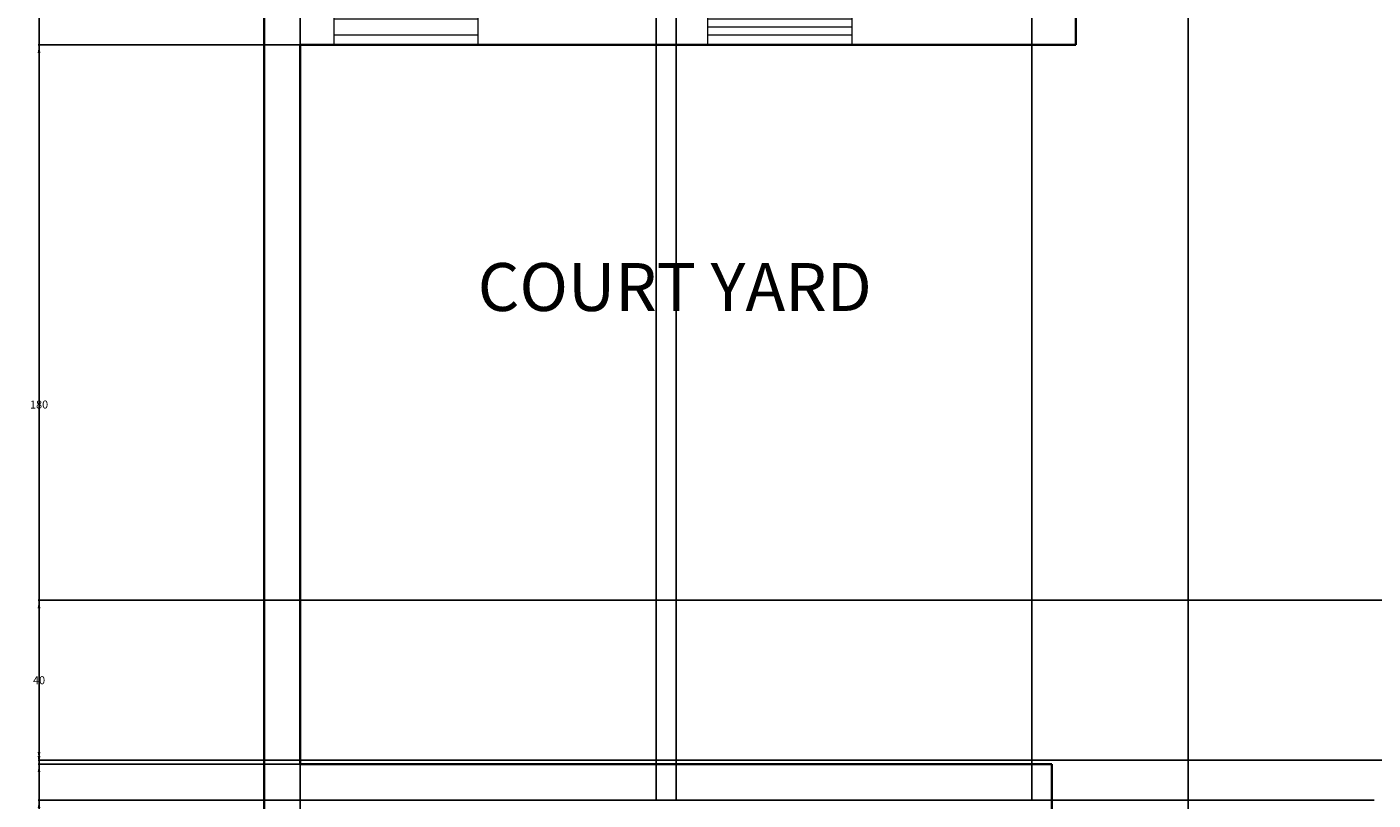
# Model space of a CAD drawing. Units: inches. Extents: x 190 to 836, y -241 to 999.
# Tile 2 of 9: x 191 to 528, y -8 to 185. Entities that reach past the tile are written whole.
import ezdxf

# ---------------------------------------------------------------- set-up
doc = ezdxf.new("R2010")
doc.units = ezdxf.units.IN
doc.header["$MEASUREMENT"] = 0
for name, color, linetype, lineweight in [('A-ANNO-DIMS', 2, 'Continuous', 18), ('A-AREA-IDEN', 7, 'Continuous', 18), ('A-GLAZ', 4, 'Continuous', 18), ('A-WALL', 7, 'Continuous', 35)]:
    doc.layers.add(name, color=color, linetype=linetype, lineweight=lineweight)
doc.styles.get("Standard").update_dxf_attribs({"font": 'arial.ttf'})
doc.dimstyles.get("Standard").update_dxf_attribs({"dimtxt": 2, "dimasz": 2, "dimexe": 0.18, "dimexo": 0.0625, "dimgap": 0.09, "dimtad": 0, "dimtih": 1, "dimtoh": 1, "dimdec": 0, "dimzin": 0, "dimdsep": 46, "dimlunit": 3, "dimtxsty": 'Standard', "dimcen": 0.09, "dimadec": 0, "dimazin": 0, "dimtfac": 1, "dimtdec": 0, "dimtofl": 0, "dimtmove": 0, "dimatfit": 3, "dimfxl": 1, "dimtolj": 1, "dimtzin": 0, "dimarcsym": 0})

# ---------------------------------------------------------------- blocks, each defined once
blk = doc.blocks.new('WIN-36IN-9IN-3LINE')
for p, q in [((2.5, 36), (2.5, 0)), ((4.5, 36), (4.5, 0)), ((6.5, 36), (6.5, 0))]:
    blk.add_line(p, q)
blk.add_lwpolyline([(0, 0), (9, 0), (9, 36), (0, 36)], close=True)
blk = doc.blocks.new('WIN-36IN-9IN-2LINE')
for p, q in [((0, 6.5), (36, 6.5)), ((0, 2.5), (36, 2.5))]:
    blk.add_line(p, q)
blk.add_lwpolyline([(36, 0), (36, 9), (0, 9), (0, 0)], close=True)
blk = doc.blocks.new('*D17')
at = {"layer": 'A-ANNO-DIMS', "color": 0, "lineweight": -2, "transparency": 16777216}
for p, q in [((250.38, 941.53), (193.96, 941.53)), ((194.14, 939.53), (194.14, 380.14)), ((194.14, -181.47), (194.14, 377.92)), ((447.38, -183.47), (193.96, -183.47))]:
    blk.add_line(p, q, dxfattribs=at)
at = {"layer": 'A-ANNO-DIMS', "color": 0, "transparency": 16777216}
for points in [[(193.8, 939.53), (194.47, 939.53), (194.14, 941.53)], [(193.8, -181.47), (194.47, -181.47), (194.14, -183.47)]]:
    blk.add_solid(points, dxfattribs=at)
at = {"layer": 'Defpoints', "color": 0, "transparency": 16777216}
for p in [(194.14, 941.53), (250.44, 941.53), (447.44, -183.47)]:
    blk.add_point(p, dxfattribs=at)
at = {"layer": 'A-ANNO-DIMS', "color": 0, "transparency": 16777216, "insert": (194.14, 379.03), "char_height": 2, "attachment_point": 5}
blk.add_mtext('\\A1;1125', dxfattribs=at)
blk = doc.blocks.new('*D29')
at = {"layer": 'A-ANNO-DIMS', "color": 0, "lineweight": -2, "transparency": 16777216}
for p, q in [((259.44, 565.47), (259.44, -239.95)), ((481.55, 565.47), (481.55, -239.95)), ((261.44, -239.77), (367.21, -239.77)), ((479.55, -239.77), (373.79, -239.77))]:
    blk.add_line(p, q, dxfattribs=at)
at = {"layer": 'A-ANNO-DIMS', "color": 0, "transparency": 16777216}
for points in [[(261.44, -239.44), (261.44, -240.11), (259.44, -239.77)], [(479.55, -239.44), (479.55, -240.11), (481.55, -239.77)]]:
    blk.add_solid(points, dxfattribs=at)
at = {"layer": 'Defpoints', "color": 0, "transparency": 16777216}
for p in [(259.44, 565.53), (481.55, 565.53), (481.55, -239.77)]:
    blk.add_point(p, dxfattribs=at)
at = {"layer": 'A-ANNO-DIMS', "color": 0, "transparency": 16777216, "insert": (370.5, -239.77), "char_height": 2, "attachment_point": 5}
blk.add_mtext('\\A1;222.1', dxfattribs=at)
blk = doc.blocks.new('*D33')
at = {"layer": 'A-ANNO-DIMS', "color": 0, "lineweight": -2, "transparency": 16777216}
for p, q in [((453.38, 180.53), (193.96, 180.53)), ((194.14, 178.53), (194.14, 91.64)), ((194.14, 2.53), (194.14, 89.42)), ((447.38, 0.53), (193.96, 0.53))]:
    blk.add_line(p, q, dxfattribs=at)
at = {"layer": 'A-ANNO-DIMS', "color": 0, "transparency": 16777216}
for points in [[(193.8, 178.53), (194.47, 178.53), (194.14, 180.53)], [(193.8, 2.53), (194.47, 2.53), (194.14, 0.53)]]:
    blk.add_solid(points, dxfattribs=at)
at = {"layer": 'Defpoints', "color": 0, "transparency": 16777216}
for p in [(194.14, 180.53), (453.44, 180.53), (447.44, 0.53)]:
    blk.add_point(p, dxfattribs=at)
at = {"layer": 'A-ANNO-DIMS', "color": 0, "transparency": 16777216, "insert": (194.14, 90.53), "char_height": 2, "attachment_point": 5}
blk.add_mtext('\\A1;180', dxfattribs=at)
blk = doc.blocks.new('*D34')
at = {"layer": 'A-ANNO-DIMS', "color": 0, "lineweight": -2, "transparency": 16777216}
for p, q in [((447.38, 0.53), (193.96, 0.53)), ((194.14, -1.47), (194.14, -67.36)), ((194.14, -135.47), (194.14, -69.58)), ((447.38, -137.47), (193.96, -137.47))]:
    blk.add_line(p, q, dxfattribs=at)
at = {"layer": 'A-ANNO-DIMS', "color": 0, "transparency": 16777216}
for points in [[(193.8, -1.47), (194.47, -1.47), (194.14, 0.53)], [(193.8, -135.47), (194.47, -135.47), (194.14, -137.47)]]:
    blk.add_solid(points, dxfattribs=at)
at = {"layer": 'Defpoints', "color": 0, "transparency": 16777216}
for p in [(194.14, 0.53), (447.44, 0.53), (447.44, -137.47)]:
    blk.add_point(p, dxfattribs=at)
at = {"layer": 'A-ANNO-DIMS', "color": 0, "transparency": 16777216, "insert": (194.14, -68.47), "char_height": 2, "attachment_point": 5}
blk.add_mtext('\\A1;138', dxfattribs=at)
blk = doc.blocks.new('*D35')
at = {"layer": 'A-ANNO-DIMS', "color": 0, "lineweight": -2, "transparency": 16777216}
for p, q in [((259.44, -8.41), (259.44, 998.02)), ((261.44, 997.84), (302.42, 997.84)), ((346.44, 997.84), (305.47, 997.84)), ((348.44, -8.41), (348.44, 998.02))]:
    blk.add_line(p, q, dxfattribs=at)
at = {"layer": 'A-ANNO-DIMS', "color": 0, "transparency": 16777216}
for points in [[(261.44, 998.17), (261.44, 997.5), (259.44, 997.84)], [(346.44, 998.17), (346.44, 997.5), (348.44, 997.84)]]:
    blk.add_solid(points, dxfattribs=at)
at = {"layer": 'Defpoints', "color": 0, "transparency": 16777216}
for p in [(348.44, 997.84), (259.44, -8.47), (348.44, -8.47)]:
    blk.add_point(p, dxfattribs=at)
at = {"layer": 'A-ANNO-DIMS', "color": 0, "transparency": 16777216, "insert": (303.94, 997.84), "char_height": 2, "attachment_point": 5}
blk.add_mtext('\\A1;89', dxfattribs=at)
blk = doc.blocks.new('*D36')
at = {"layer": 'A-ANNO-DIMS', "color": 0, "lineweight": -2, "transparency": 16777216}
for p, q in [((353.44, -8.41), (353.44, 998.02)), ((355.44, 997.84), (396.42, 997.84)), ((440.44, 997.84), (399.47, 997.84)), ((442.44, -8.41), (442.44, 998.02))]:
    blk.add_line(p, q, dxfattribs=at)
at = {"layer": 'A-ANNO-DIMS', "color": 0, "transparency": 16777216}
for points in [[(355.44, 998.17), (355.44, 997.5), (353.44, 997.84)], [(440.44, 998.17), (440.44, 997.5), (442.44, 997.84)]]:
    blk.add_solid(points, dxfattribs=at)
at = {"layer": 'Defpoints', "color": 0, "transparency": 16777216}
for p in [(442.44, 997.84), (353.44, -8.47), (442.44, -8.47)]:
    blk.add_point(p, dxfattribs=at)
at = {"layer": 'A-ANNO-DIMS', "color": 0, "transparency": 16777216, "insert": (397.94, 997.84), "char_height": 2, "attachment_point": 5}
blk.add_mtext('\\A1;89', dxfattribs=at)
blk = doc.blocks.new('*D40')
at = {"layer": 'A-ANNO-DIMS', "color": 0, "lineweight": -2, "transparency": 16777216}
for p, q in [((528.04, -8.47), (193.96, -8.47)), ((194.14, -10.47), (194.14, -67.36)), ((194.14, -126.47), (194.14, -69.58)), ((533.04, -128.47), (193.96, -128.47))]:
    blk.add_line(p, q, dxfattribs=at)
at = {"layer": 'A-ANNO-DIMS', "color": 0, "transparency": 16777216}
for points in [[(193.8, -10.47), (194.47, -10.47), (194.14, -8.47)], [(193.8, -126.47), (194.47, -126.47), (194.14, -128.47)]]:
    blk.add_solid(points, dxfattribs=at)
at = {"layer": 'Defpoints', "color": 0, "transparency": 16777216}
for p in [(194.14, -8.47), (528.1, -8.47), (533.1, -128.47)]:
    blk.add_point(p, dxfattribs=at)
at = {"layer": 'A-ANNO-DIMS', "color": 0, "transparency": 16777216, "insert": (194.14, -68.47), "char_height": 2, "attachment_point": 5}
blk.add_mtext('\\A1;120', dxfattribs=at)
blk = doc.blocks.new('*D49')
at = {"layer": 'A-ANNO-DIMS', "color": 0, "lineweight": -2, "transparency": 16777216}
for p, q in [((607.04, 41.53), (193.96, 41.53)), ((194.14, 39.53), (194.14, 22.64)), ((194.14, 3.53), (194.14, 20.42)), ((606.04, 1.53), (193.96, 1.53))]:
    blk.add_line(p, q, dxfattribs=at)
at = {"layer": 'A-ANNO-DIMS', "color": 0, "transparency": 16777216}
for points in [[(193.8, 39.53), (194.47, 39.53), (194.14, 41.53)], [(193.8, 3.53), (194.47, 3.53), (194.14, 1.53)]]:
    blk.add_solid(points, dxfattribs=at)
at = {"layer": 'Defpoints', "color": 0, "transparency": 16777216}
for p in [(607.1, 41.53), (194.14, 1.53), (606.1, 1.53)]:
    blk.add_point(p, dxfattribs=at)
at = {"layer": 'A-ANNO-DIMS', "color": 0, "transparency": 16777216, "insert": (194.14, 21.53), "char_height": 2, "attachment_point": 5}
blk.add_mtext('\\A1;40', dxfattribs=at)

msp = doc.modelspace()

# ---------------------------------------------------------------- linework, layer by layer
at = {"layer": 'A-WALL'}
for p, q in [((250.4421, -137.4687), (250.4421, 565.5313)), ((453.4421, 342.5313), (453.4421, 180.5313)), ((453.4421, 180.5313), (259.4421, 180.5313)), ((259.4421, 0.5313), (259.4421, 180.5313)), ((447.4421, 0.5313), (259.4421, 0.5313)), ((447.4421, -137.4687), (447.4421, 0.5313))]:
    msp.add_line(p, q, dxfattribs=at)

# ---------------------------------------------------------------- block references
at = {"layer": 'A-GLAZ', "extrusion": (0, 0, -1), "zscale": -1}
for name, p, rotation in [('WIN-36IN-9IN-2LINE', (-267.917, 189.5317), 180), ('WIN-36IN-9IN-3LINE', (-397.4358, 189.5315), 269.9999999999998)]:
    msp.add_blockref(name, p, dxfattribs=dict(at, rotation=rotation))

# ---------------------------------------------------------------- texts
at = {"layer": 'A-AREA-IDEN', "insert": (303.8416, 125.9353), "char_height": 12, "attachment_point": 1}
msp.add_mtext_dynamic_manual_height_columns('COURT YARD', width=145.957398, gutter_width=1, heights=[0], dxfattribs=at)

# ---------------------------------------------------------------- dimensions: what is measured, and where the dimension line sits
at = {"layer": 'A-ANNO-DIMS'}
for base, p1, p2, override, picture, middle in [((348.4421, 997.8363), (259.4421, -8.4687), (348.4421, -8.4687), {"dimdec": 0, "dimlfac": 1, "dimrnd": 0, "dimzin": 0, "dimdsep": 46, "dimlunit": 2}, '*D35', (303.9421, 997.8363)), ((442.4421, 997.8363), (353.4421, -8.4687), (442.4421, -8.4687), {"dimdec": 0, "dimlfac": 1, "dimrnd": 0, "dimzin": 0, "dimdsep": 46, "dimlunit": 2}, '*D36', (397.9421, 997.8363)), ((481.5536, -239.7737), (259.4421, 565.5313), (481.5536, 565.5313), {"dimdec": 1, "dimlfac": 1, "dimrnd": 0, "dimzin": 0, "dimdsep": 46, "dimlunit": 2}, '*D29', (370.4979, -239.7737))]:
    dim = msp.add_linear_dim(base=base, p1=p1, p2=p2, dimstyle='Standard', override=override, dxfattribs=at)
    dim.commit()
    dim.dimension.update_dxf_attribs({"geometry": picture, "text_midpoint": middle})
for base, p1, p2, picture, middle in [((194.1371, 941.5313), (447.4421, -183.4687), (250.4421, 941.5313), '*D17', (194.1371, 379.0313)), ((194.1371, 180.5313), (447.4421, 0.5313), (453.4421, 180.5313), '*D33', (194.1371, 90.5313)), ((194.1371, 1.5313), (607.0998, 41.5313), (606.0998, 1.5313), '*D49', (194.1371, 21.5313)), ((194.1371, 0.5313), (447.4421, -137.4687), (447.4421, 0.5313), '*D34', (194.1371, -68.4687)), ((194.1371, -8.4687), (533.0998, -128.4687), (528.0998, -8.4687), '*D40', (194.1371, -68.4687))]:
    dim = msp.add_linear_dim(base=base, p1=p1, p2=p2, angle=90, dimstyle='Standard', override={"dimdec": 0, "dimlfac": 1, "dimrnd": 0, "dimzin": 0, "dimdsep": 46, "dimlunit": 2}, dxfattribs=at)
    dim.commit()
    dim.dimension.update_dxf_attribs({"geometry": picture, "text_midpoint": middle})

doc.saveas('drawing.dxf')
